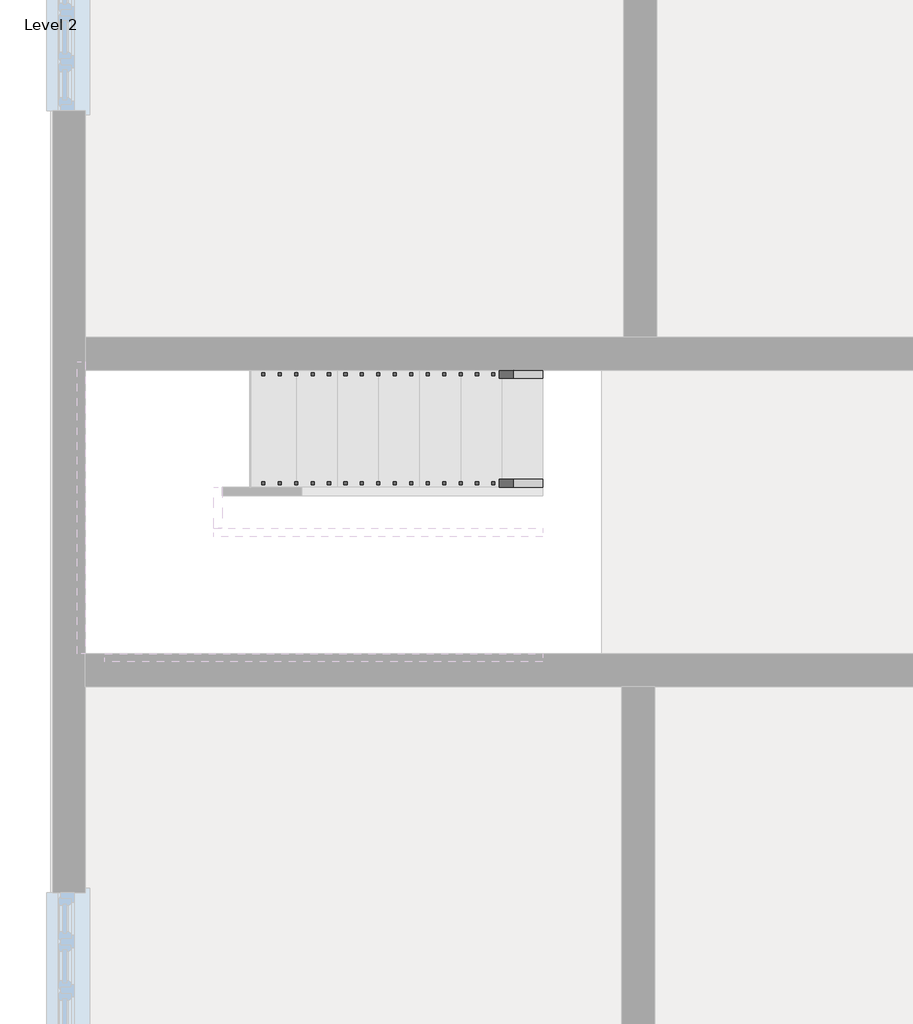
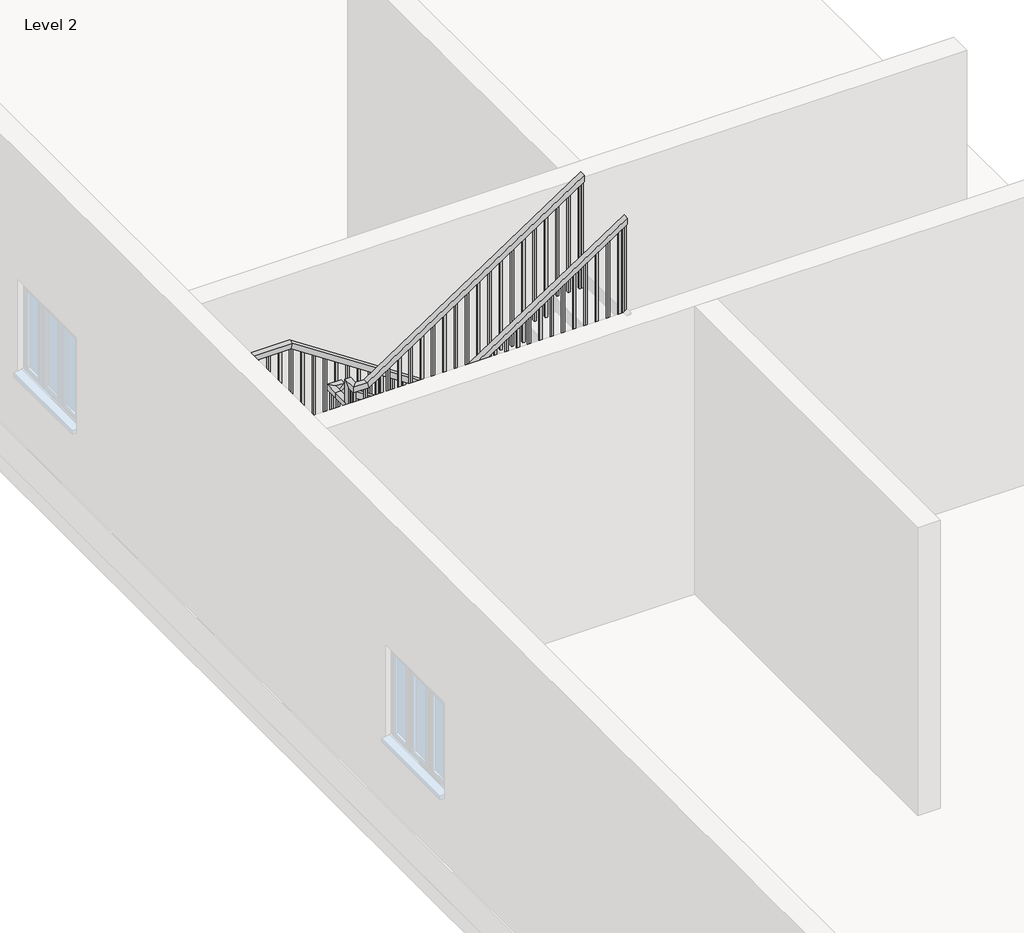
# One storey, part 2 of 3: 2 railings.
"""IFC4 building model written with IfcOpenShell, lengths in millimetres."""

from ifc_helpers import new_model, si_unit, frame, origin, place, context, project, spatial, polyline, outline, extrude, faceted_brep, element, save

model = new_model("IFC4")

# Units and contexts
model_context = context("Model", 3, world=origin())
ifc_project = project(units=[si_unit("LENGTHUNIT", "METRE", prefix="MILLI")], contexts=[model_context])

# Site, building, storey
site = spatial("IfcSite", under=ifc_project)
building = spatial("IfcBuilding", under=site)
storey = spatial("IfcBuildingStorey", under=building, Name="Level 2", Elevation=3048.0)

# Railings
placement = place(None, origin())
element("IfcRailing", 1, ObjectType="Handrail - Rectangular", at=placement, inside=storey, context=model_context, shape_type="SolidModel", body=[
    faceted_brep([(-2118.1728655, 1141.7797121, 4130.3222222), (-2118.1728655, 1141.7797121, 4069.4243166), (-2118.1728655, 1192.5797121, 4069.4243166), (-2118.1728655, 1192.5797121, 4130.3222222), (-4150.1728655, 1141.7797121, 5473.7), (-4165.4470084, 1141.7797121, 5422.9), (-4165.4470084, 1192.5797121, 5422.9), (-4150.1728655, 1192.5797121, 5473.7), (-4893.1394105, 1141.7797121, 5473.7), (-4893.1394105, 1141.7797121, 5422.9), (-4943.9394105, 1192.5797121, 5422.9), (-4943.9394105, 1192.5797121, 5473.7), (-4893.1394105, -509.2202879, 5473.7), (-4893.1394105, -509.2202879, 5422.9), (-4943.9394105, -560.0202879, 5422.9), (-4943.9394105, -560.0202879, 5473.7), (-4404.1728655, -509.2202879, 5473.7), (-4388.8987225, -509.2202879, 5422.9), (-4388.8987225, -560.0202879, 5422.9), (-4404.1728655, -560.0202879, 5473.7), (-2118.1728655, -509.2202879, 6985.0), (-2118.1728655, -560.0202879, 6985.0), (-2118.1728655, -560.0202879, 6924.1020944), (-2118.1728655, -509.2202879, 6924.1020944)], [[[0, 1, 2, 3]], [[1, 0, 4, 5]], [[2, 1, 5, 6]], [[3, 2, 6, 7]], [[0, 3, 7, 4]], [[5, 4, 8, 9]], [[6, 5, 9, 10]], [[7, 6, 10, 11]], [[4, 7, 11, 8]], [[9, 8, 12, 13]], [[10, 9, 13, 14]], [[11, 10, 14, 15]], [[8, 11, 15, 12]], [[13, 12, 16, 17]], [[14, 13, 17, 18]], [[15, 14, 18, 19]], [[12, 15, 19, 16]], [[20, 21, 22, 23]], [[17, 16, 20, 23]], [[18, 17, 23, 22]], [[19, 18, 22, 21]], [[16, 19, 21, 20]]]),
    extrude(outline(polyline([(6892.6057396, -2165.8144105), (6880.0115729, -2184.8644105), (5902.6777778, -2184.8644105), (5902.6777778, -2165.8144105), (6892.6057396, -2165.8144105)])), frame((0.0, -544.1452879, 0.0), z_axis=(0.0, 1.0, 0.0), x_axis=(0.0, 0.0, 1.0)), (0.0, 0.0, 1.0), 19.05),
    extrude(outline(polyline([(6825.4368507, -2267.4144105), (6812.842684, -2286.4644105), (5902.6777778, -2286.4644105), (5902.6777778, -2267.4144105), (6825.4368507, -2267.4144105)])), frame((0.0, -544.1452879, 0.0), z_axis=(0.0, 1.0, 0.0), x_axis=(0.0, 0.0, 1.0)), (0.0, 0.0, 1.0), 19.05),
    extrude(outline(polyline([(6758.2679618, -2369.0144105), (6745.6737951, -2388.0644105), (5734.7555556, -2388.0644105), (5734.7555556, -2369.0144105), (6758.2679618, -2369.0144105)])), frame((0.0, -544.1452879, 0.0), z_axis=(0.0, 1.0, 0.0), x_axis=(0.0, 0.0, 1.0)), (0.0, 0.0, 1.0), 19.05),
    extrude(outline(polyline([(6691.0990729, -2470.6144105), (6678.5049062, -2489.6644105), (5734.7555556, -2489.6644105), (5734.7555556, -2470.6144105), (6691.0990729, -2470.6144105)])), frame((0.0, -544.1452879, 0.0), z_axis=(0.0, 1.0, 0.0), x_axis=(0.0, 0.0, 1.0)), (0.0, 0.0, 1.0), 19.05),
    extrude(outline(polyline([(6623.930184, -2572.2144105), (6611.3360174, -2591.2644105), (5734.7555556, -2591.2644105), (5734.7555556, -2572.2144105), (6623.930184, -2572.2144105)])), frame((0.0, -544.1452879, 0.0), z_axis=(0.0, 1.0, 0.0), x_axis=(0.0, 0.0, 1.0)), (0.0, 0.0, 1.0), 19.05),
    extrude(outline(polyline([(6556.7612951, -2673.8144105), (6544.1671285, -2692.8644105), (5566.8333333, -2692.8644105), (5566.8333333, -2673.8144105), (6556.7612951, -2673.8144105)])), frame((0.0, -544.1452879, 0.0), z_axis=(0.0, 1.0, 0.0), x_axis=(0.0, 0.0, 1.0)), (0.0, 0.0, 1.0), 19.05),
    extrude(outline(polyline([(6489.5924062, -2775.4144105), (6476.9982396, -2794.4644105), (5566.8333333, -2794.4644105), (5566.8333333, -2775.4144105), (6489.5924062, -2775.4144105)])), frame((0.0, -544.1452879, 0.0), z_axis=(0.0, 1.0, 0.0), x_axis=(0.0, 0.0, 1.0)), (0.0, 0.0, 1.0), 19.05),
    extrude(outline(polyline([(6422.4235174, -2877.0144105), (6409.8293507, -2896.0644105), (5398.9111111, -2896.0644105), (5398.9111111, -2877.0144105), (6422.4235174, -2877.0144105)])), frame((0.0, -544.1452879, 0.0), z_axis=(0.0, 1.0, 0.0), x_axis=(0.0, 0.0, 1.0)), (0.0, 0.0, 1.0), 19.05),
    extrude(outline(polyline([(6355.2546285, -2978.6144105), (6342.6604618, -2997.6644105), (5398.9111111, -2997.6644105), (5398.9111111, -2978.6144105), (6355.2546285, -2978.6144105)])), frame((0.0, -544.1452879, 0.0), z_axis=(0.0, 1.0, 0.0), x_axis=(0.0, 0.0, 1.0)), (0.0, 0.0, 1.0), 19.05),
    extrude(outline(polyline([(6288.0857396, -3080.2144105), (6275.4915729, -3099.2644105), (5398.9111111, -3099.2644105), (5398.9111111, -3080.2144105), (6288.0857396, -3080.2144105)])), frame((0.0, -544.1452879, 0.0), z_axis=(0.0, 1.0, 0.0), x_axis=(0.0, 0.0, 1.0)), (0.0, 0.0, 1.0), 19.05),
    extrude(outline(polyline([(6220.9168507, -3181.8144105), (6208.322684, -3200.8644105), (5230.9888889, -3200.8644105), (5230.9888889, -3181.8144105), (6220.9168507, -3181.8144105)])), frame((0.0, -544.1452879, 0.0), z_axis=(0.0, 1.0, 0.0), x_axis=(0.0, 0.0, 1.0)), (0.0, 0.0, 1.0), 19.05),
    extrude(outline(polyline([(6153.7479618, -3283.4144105), (6141.1537951, -3302.4644105), (5230.9888889, -3302.4644105), (5230.9888889, -3283.4144105), (6153.7479618, -3283.4144105)])), frame((0.0, -544.1452879, 0.0), z_axis=(0.0, 1.0, 0.0), x_axis=(0.0, 0.0, 1.0)), (0.0, 0.0, 1.0), 19.05),
    extrude(outline(polyline([(6086.5790729, -3385.0144105), (6073.9849062, -3404.0644105), (5063.0666667, -3404.0644105), (5063.0666667, -3385.0144105), (6086.5790729, -3385.0144105)])), frame((0.0, -544.1452879, 0.0), z_axis=(0.0, 1.0, 0.0), x_axis=(0.0, 0.0, 1.0)), (0.0, 0.0, 1.0), 19.05),
    extrude(outline(polyline([(6019.410184, -3486.6144105), (6006.8160174, -3505.6644105), (5063.0666667, -3505.6644105), (5063.0666667, -3486.6144105), (6019.410184, -3486.6144105)])), frame((0.0, -544.1452879, 0.0), z_axis=(0.0, 1.0, 0.0), x_axis=(0.0, 0.0, 1.0)), (0.0, 0.0, 1.0), 19.05),
    extrude(outline(polyline([(5952.2412951, -3588.2144105), (5939.6471285, -3607.2644105), (5063.0666667, -3607.2644105), (5063.0666667, -3588.2144105), (5952.2412951, -3588.2144105)])), frame((0.0, -544.1452879, 0.0), z_axis=(0.0, 1.0, 0.0), x_axis=(0.0, 0.0, 1.0)), (0.0, 0.0, 1.0), 19.05),
    extrude(outline(polyline([(5885.0724062, -3689.8144105), (5872.4782396, -3708.8644105), (4895.1444444, -3708.8644105), (4895.1444444, -3689.8144105), (5885.0724062, -3689.8144105)])), frame((0.0, -544.1452879, 0.0), z_axis=(0.0, 1.0, 0.0), x_axis=(0.0, 0.0, 1.0)), (0.0, 0.0, 1.0), 19.05),
    extrude(outline(polyline([(5817.9035174, -3791.4144105), (5805.3093507, -3810.4644105), (4895.1444444, -3810.4644105), (4895.1444444, -3791.4144105), (5817.9035174, -3791.4144105)])), frame((0.0, -544.1452879, 0.0), z_axis=(0.0, 1.0, 0.0), x_axis=(0.0, 0.0, 1.0)), (0.0, 0.0, 1.0), 19.05),
    extrude(outline(polyline([(5750.7346285, -3893.0144105), (5738.1404618, -3912.0644105), (4727.2222222, -3912.0644105), (4727.2222222, -3893.0144105), (5750.7346285, -3893.0144105)])), frame((0.0, -544.1452879, 0.0), z_axis=(0.0, 1.0, 0.0), x_axis=(0.0, 0.0, 1.0)), (0.0, 0.0, 1.0), 19.05),
    extrude(outline(polyline([(5683.5657396, -3994.6144105), (5670.9715729, -4013.6644105), (4727.2222222, -4013.6644105), (4727.2222222, -3994.6144105), (5683.5657396, -3994.6144105)])), frame((0.0, -544.1452879, 0.0), z_axis=(0.0, 1.0, 0.0), x_axis=(0.0, 0.0, 1.0)), (0.0, 0.0, 1.0), 19.05),
    extrude(outline(polyline([(5616.3968507, -4096.2144105), (5603.802684, -4115.2644105), (4727.2222222, -4115.2644105), (4727.2222222, -4096.2144105), (5616.3968507, -4096.2144105)])), frame((0.0, -544.1452879, 0.0), z_axis=(0.0, 1.0, 0.0), x_axis=(0.0, 0.0, 1.0)), (0.0, 0.0, 1.0), 19.05),
    extrude(outline(polyline([(5549.2279618, -4197.8144105), (5536.6337951, -4216.8644105), (4559.3, -4216.8644105), (4559.3, -4197.8144105), (5549.2279618, -4197.8144105)])), frame((0.0, -544.1452879, 0.0), z_axis=(0.0, 1.0, 0.0), x_axis=(0.0, 0.0, 1.0)), (0.0, 0.0, 1.0), 19.05),
    extrude(outline(polyline([(5482.0590729, -4299.4144105), (5469.4649062, -4318.4644105), (4559.3, -4318.4644105), (4559.3, -4299.4144105), (5482.0590729, -4299.4144105)])), frame((0.0, -544.1452879, 0.0), z_axis=(0.0, 1.0, 0.0), x_axis=(0.0, 0.0, 1.0)), (0.0, 0.0, 1.0), 19.05),
    extrude(outline(polyline([(-4420.0644105, -544.1452879), (-4420.0644105, -525.0952879), (-4401.0144105, -525.0952879), (-4401.0144105, -544.1452879), (-4420.0644105, -544.1452879)])), frame((0.0, 0.0, 4559.3), z_axis=(0.0, 0.0, 1.0), x_axis=(1.0, 0.0, 0.0)), (0.0, 0.0, 1.0), 863.6),
    extrude(outline(polyline([(-4521.6644105, -544.1452879), (-4521.6644105, -525.0952879), (-4502.6144105, -525.0952879), (-4502.6144105, -544.1452879), (-4521.6644105, -544.1452879)])), frame((0.0, 0.0, 4559.3), z_axis=(0.0, 0.0, 1.0), x_axis=(1.0, 0.0, 0.0)), (0.0, 0.0, 1.0), 863.6),
    extrude(outline(polyline([(-4623.2644105, -544.1452879), (-4623.2644105, -525.0952879), (-4604.2144105, -525.0952879), (-4604.2144105, -544.1452879), (-4623.2644105, -544.1452879)])), frame((0.0, 0.0, 4559.3), z_axis=(0.0, 0.0, 1.0), x_axis=(1.0, 0.0, 0.0)), (0.0, 0.0, 1.0), 863.6),
    extrude(outline(polyline([(-4724.8644105, -544.1452879), (-4724.8644105, -525.0952879), (-4705.8144105, -525.0952879), (-4705.8144105, -544.1452879), (-4724.8644105, -544.1452879)])), frame((0.0, 0.0, 4559.3), z_axis=(0.0, 0.0, 1.0), x_axis=(1.0, 0.0, 0.0)), (0.0, 0.0, 1.0), 863.6),
    extrude(outline(polyline([(-4826.4644105, -544.1452879), (-4826.4644105, -525.0952879), (-4807.4144105, -525.0952879), (-4807.4144105, -544.1452879), (-4826.4644105, -544.1452879)])), frame((0.0, 0.0, 4559.3), z_axis=(0.0, 0.0, 1.0), x_axis=(1.0, 0.0, 0.0)), (0.0, 0.0, 1.0), 863.6),
    extrude(outline(polyline([(-4928.0644105, -448.8952879), (-4909.0144105, -448.8952879), (-4909.0144105, -467.9452879), (-4928.0644105, -467.9452879), (-4928.0644105, -448.8952879)])), frame((0.0, 0.0, 4559.3), z_axis=(0.0, 0.0, 1.0), x_axis=(1.0, 0.0, 0.0)), (0.0, 0.0, 1.0), 863.6),
    extrude(outline(polyline([(-4928.0644105, -347.2952879), (-4909.0144105, -347.2952879), (-4909.0144105, -366.3452879), (-4928.0644105, -366.3452879), (-4928.0644105, -347.2952879)])), frame((0.0, 0.0, 4559.3), z_axis=(0.0, 0.0, 1.0), x_axis=(1.0, 0.0, 0.0)), (0.0, 0.0, 1.0), 863.6),
    extrude(outline(polyline([(-4928.0644105, -245.6952879), (-4909.0144105, -245.6952879), (-4909.0144105, -264.7452879), (-4928.0644105, -264.7452879), (-4928.0644105, -245.6952879)])), frame((0.0, 0.0, 4559.3), z_axis=(0.0, 0.0, 1.0), x_axis=(1.0, 0.0, 0.0)), (0.0, 0.0, 1.0), 863.6),
    extrude(outline(polyline([(-4928.0644105, -144.0952879), (-4909.0144105, -144.0952879), (-4909.0144105, -163.1452879), (-4928.0644105, -163.1452879), (-4928.0644105, -144.0952879)])), frame((0.0, 0.0, 4559.3), z_axis=(0.0, 0.0, 1.0), x_axis=(1.0, 0.0, 0.0)), (0.0, 0.0, 1.0), 863.6),
    extrude(outline(polyline([(-4928.0644105, -42.4952879), (-4909.0144105, -42.4952879), (-4909.0144105, -61.5452879), (-4928.0644105, -61.5452879), (-4928.0644105, -42.4952879)])), frame((0.0, 0.0, 4559.3), z_axis=(0.0, 0.0, 1.0), x_axis=(1.0, 0.0, 0.0)), (0.0, 0.0, 1.0), 863.6),
    extrude(outline(polyline([(-4928.0644105, 59.1047121), (-4909.0144105, 59.1047121), (-4909.0144105, 40.0547121), (-4928.0644105, 40.0547121), (-4928.0644105, 59.1047121)])), frame((0.0, 0.0, 4559.3), z_axis=(0.0, 0.0, 1.0), x_axis=(1.0, 0.0, 0.0)), (0.0, 0.0, 1.0), 863.6),
    extrude(outline(polyline([(-4928.0644105, 160.7047121), (-4909.0144105, 160.7047121), (-4909.0144105, 141.6547121), (-4928.0644105, 141.6547121), (-4928.0644105, 160.7047121)])), frame((0.0, 0.0, 4559.3), z_axis=(0.0, 0.0, 1.0), x_axis=(1.0, 0.0, 0.0)), (0.0, 0.0, 1.0), 863.6),
    extrude(outline(polyline([(-4928.0644105, 262.3047121), (-4909.0144105, 262.3047121), (-4909.0144105, 243.2547121), (-4928.0644105, 243.2547121), (-4928.0644105, 262.3047121)])), frame((0.0, 0.0, 4559.3), z_axis=(0.0, 0.0, 1.0), x_axis=(1.0, 0.0, 0.0)), (0.0, 0.0, 1.0), 863.6),
    extrude(outline(polyline([(-4928.0644105, 363.9047121), (-4909.0144105, 363.9047121), (-4909.0144105, 344.8547121), (-4928.0644105, 344.8547121), (-4928.0644105, 363.9047121)])), frame((0.0, 0.0, 4559.3), z_axis=(0.0, 0.0, 1.0), x_axis=(1.0, 0.0, 0.0)), (0.0, 0.0, 1.0), 863.6),
    extrude(outline(polyline([(-4928.0644105, 465.5047121), (-4909.0144105, 465.5047121), (-4909.0144105, 446.4547121), (-4928.0644105, 446.4547121), (-4928.0644105, 465.5047121)])), frame((0.0, 0.0, 4559.3), z_axis=(0.0, 0.0, 1.0), x_axis=(1.0, 0.0, 0.0)), (0.0, 0.0, 1.0), 863.6),
    extrude(outline(polyline([(-4928.0644105, 567.1047121), (-4909.0144105, 567.1047121), (-4909.0144105, 548.0547121), (-4928.0644105, 548.0547121), (-4928.0644105, 567.1047121)])), frame((0.0, 0.0, 4559.3), z_axis=(0.0, 0.0, 1.0), x_axis=(1.0, 0.0, 0.0)), (0.0, 0.0, 1.0), 863.6),
    extrude(outline(polyline([(-4928.0644105, 668.7047121), (-4909.0144105, 668.7047121), (-4909.0144105, 649.6547121), (-4928.0644105, 649.6547121), (-4928.0644105, 668.7047121)])), frame((0.0, 0.0, 4559.3), z_axis=(0.0, 0.0, 1.0), x_axis=(1.0, 0.0, 0.0)), (0.0, 0.0, 1.0), 863.6),
    extrude(outline(polyline([(-4928.0644105, 770.3047121), (-4909.0144105, 770.3047121), (-4909.0144105, 751.2547121), (-4928.0644105, 751.2547121), (-4928.0644105, 770.3047121)])), frame((0.0, 0.0, 4559.3), z_axis=(0.0, 0.0, 1.0), x_axis=(1.0, 0.0, 0.0)), (0.0, 0.0, 1.0), 863.6),
    extrude(outline(polyline([(-4928.0644105, 871.9047121), (-4909.0144105, 871.9047121), (-4909.0144105, 852.8547121), (-4928.0644105, 852.8547121), (-4928.0644105, 871.9047121)])), frame((0.0, 0.0, 4559.3), z_axis=(0.0, 0.0, 1.0), x_axis=(1.0, 0.0, 0.0)), (0.0, 0.0, 1.0), 863.6),
    extrude(outline(polyline([(-4928.0644105, 973.5047121), (-4909.0144105, 973.5047121), (-4909.0144105, 954.4547121), (-4928.0644105, 954.4547121), (-4928.0644105, 973.5047121)])), frame((0.0, 0.0, 4559.3), z_axis=(0.0, 0.0, 1.0), x_axis=(1.0, 0.0, 0.0)), (0.0, 0.0, 1.0), 863.6),
    extrude(outline(polyline([(-4928.0644105, 1075.1047121), (-4909.0144105, 1075.1047121), (-4909.0144105, 1056.0547121), (-4928.0644105, 1056.0547121), (-4928.0644105, 1075.1047121)])), frame((0.0, 0.0, 4559.3), z_axis=(0.0, 0.0, 1.0), x_axis=(1.0, 0.0, 0.0)), (0.0, 0.0, 1.0), 863.6),
    extrude(outline(polyline([(-4851.8478655, 1176.7047121), (-4851.8478655, 1157.6547121), (-4870.8978655, 1157.6547121), (-4870.8978655, 1176.7047121), (-4851.8478655, 1176.7047121)])), frame((0.0, 0.0, 4559.3), z_axis=(0.0, 0.0, 1.0), x_axis=(1.0, 0.0, 0.0)), (0.0, 0.0, 1.0), 863.6),
    extrude(outline(polyline([(-4750.2478655, 1176.7047121), (-4750.2478655, 1157.6547121), (-4769.2978655, 1157.6547121), (-4769.2978655, 1176.7047121), (-4750.2478655, 1176.7047121)])), frame((0.0, 0.0, 4559.3), z_axis=(0.0, 0.0, 1.0), x_axis=(1.0, 0.0, 0.0)), (0.0, 0.0, 1.0), 863.6),
    extrude(outline(polyline([(-4648.6478655, 1176.7047121), (-4648.6478655, 1157.6547121), (-4667.6978655, 1157.6547121), (-4667.6978655, 1176.7047121), (-4648.6478655, 1176.7047121)])), frame((0.0, 0.0, 4559.3), z_axis=(0.0, 0.0, 1.0), x_axis=(1.0, 0.0, 0.0)), (0.0, 0.0, 1.0), 863.6),
    extrude(outline(polyline([(-4547.0478655, 1176.7047121), (-4547.0478655, 1157.6547121), (-4566.0978655, 1157.6547121), (-4566.0978655, 1176.7047121), (-4547.0478655, 1176.7047121)])), frame((0.0, 0.0, 4559.3), z_axis=(0.0, 0.0, 1.0), x_axis=(1.0, 0.0, 0.0)), (0.0, 0.0, 1.0), 863.6),
    extrude(outline(polyline([(-4445.4478655, 1176.7047121), (-4445.4478655, 1157.6547121), (-4464.4978655, 1157.6547121), (-4464.4978655, 1176.7047121), (-4445.4478655, 1176.7047121)])), frame((0.0, 0.0, 4559.3), z_axis=(0.0, 0.0, 1.0), x_axis=(1.0, 0.0, 0.0)), (0.0, 0.0, 1.0), 863.6),
    extrude(outline(polyline([(-4343.8478655, 1176.7047121), (-4343.8478655, 1157.6547121), (-4362.8978655, 1157.6547121), (-4362.8978655, 1176.7047121), (-4343.8478655, 1176.7047121)])), frame((0.0, 0.0, 4559.3), z_axis=(0.0, 0.0, 1.0), x_axis=(1.0, 0.0, 0.0)), (0.0, 0.0, 1.0), 863.6),
    extrude(outline(polyline([(-4242.2478655, 1176.7047121), (-4242.2478655, 1157.6547121), (-4261.2978655, 1157.6547121), (-4261.2978655, 1176.7047121), (-4242.2478655, 1176.7047121)])), frame((0.0, 0.0, 4559.3), z_axis=(0.0, 0.0, 1.0), x_axis=(1.0, 0.0, 0.0)), (0.0, 0.0, 1.0), 863.6),
    extrude(outline(polyline([(5406.505011, -4140.6478655), (5419.0991777, -4159.6978655), (4559.3, -4159.6978655), (4559.3, -4140.6478655), (5406.505011, -4140.6478655)])), frame((0.0, 1157.6547121, 0.0), z_axis=(0.0, 1.0, 0.0), x_axis=(0.0, 0.0, 1.0)), (0.0, 0.0, 1.0), 19.05),
    extrude(outline(polyline([(5339.3361222, -4039.0478655), (5351.9302888, -4058.0978655), (4391.3777778, -4058.0978655), (4391.3777778, -4039.0478655), (5339.3361222, -4039.0478655)])), frame((0.0, 1157.6547121, 0.0), z_axis=(0.0, 1.0, 0.0), x_axis=(0.0, 0.0, 1.0)), (0.0, 0.0, 1.0), 19.05),
    extrude(outline(polyline([(5272.1672333, -3937.4478655), (5284.7613999, -3956.4978655), (4391.3777778, -3956.4978655), (4391.3777778, -3937.4478655), (5272.1672333, -3937.4478655)])), frame((0.0, 1157.6547121, 0.0), z_axis=(0.0, 1.0, 0.0), x_axis=(0.0, 0.0, 1.0)), (0.0, 0.0, 1.0), 19.05),
    extrude(outline(polyline([(5204.9983444, -3835.8478655), (5217.592511, -3854.8978655), (4223.4555556, -3854.8978655), (4223.4555556, -3835.8478655), (5204.9983444, -3835.8478655)])), frame((0.0, 1157.6547121, 0.0), z_axis=(0.0, 1.0, 0.0), x_axis=(0.0, 0.0, 1.0)), (0.0, 0.0, 1.0), 19.05),
    extrude(outline(polyline([(5137.8294555, -3734.2478655), (5150.4236222, -3753.2978655), (4223.4555556, -3753.2978655), (4223.4555556, -3734.2478655), (5137.8294555, -3734.2478655)])), frame((0.0, 1157.6547121, 0.0), z_axis=(0.0, 1.0, 0.0), x_axis=(0.0, 0.0, 1.0)), (0.0, 0.0, 1.0), 19.05),
    extrude(outline(polyline([(5070.6605666, -3632.6478655), (5083.2547333, -3651.6978655), (4223.4555556, -3651.6978655), (4223.4555556, -3632.6478655), (5070.6605666, -3632.6478655)])), frame((0.0, 1157.6547121, 0.0), z_axis=(0.0, 1.0, 0.0), x_axis=(0.0, 0.0, 1.0)), (0.0, 0.0, 1.0), 19.05),
    extrude(outline(polyline([(5003.4916777, -3531.0478655), (5016.0858444, -3550.0978655), (4055.5333333, -3550.0978655), (4055.5333333, -3531.0478655), (5003.4916777, -3531.0478655)])), frame((0.0, 1157.6547121, 0.0), z_axis=(0.0, 1.0, 0.0), x_axis=(0.0, 0.0, 1.0)), (0.0, 0.0, 1.0), 19.05),
    extrude(outline(polyline([(4936.3227888, -3429.4478655), (4948.9169555, -3448.4978655), (4055.5333333, -3448.4978655), (4055.5333333, -3429.4478655), (4936.3227888, -3429.4478655)])), frame((0.0, 1157.6547121, 0.0), z_axis=(0.0, 1.0, 0.0), x_axis=(0.0, 0.0, 1.0)), (0.0, 0.0, 1.0), 19.05),
    extrude(outline(polyline([(4869.1538999, -3327.8478655), (4881.7480666, -3346.8978655), (3887.6111111, -3346.8978655), (3887.6111111, -3327.8478655), (4869.1538999, -3327.8478655)])), frame((0.0, 1157.6547121, 0.0), z_axis=(0.0, 1.0, 0.0), x_axis=(0.0, 0.0, 1.0)), (0.0, 0.0, 1.0), 19.05),
    extrude(outline(polyline([(4801.985011, -3226.2478655), (4814.5791777, -3245.2978655), (3887.6111111, -3245.2978655), (3887.6111111, -3226.2478655), (4801.985011, -3226.2478655)])), frame((0.0, 1157.6547121, 0.0), z_axis=(0.0, 1.0, 0.0), x_axis=(0.0, 0.0, 1.0)), (0.0, 0.0, 1.0), 19.05),
    extrude(outline(polyline([(4734.8161222, -3124.6478655), (4747.4102888, -3143.6978655), (3887.6111111, -3143.6978655), (3887.6111111, -3124.6478655), (4734.8161222, -3124.6478655)])), frame((0.0, 1157.6547121, 0.0), z_axis=(0.0, 1.0, 0.0), x_axis=(0.0, 0.0, 1.0)), (0.0, 0.0, 1.0), 19.05),
    extrude(outline(polyline([(4667.6472333, -3023.0478655), (4680.2413999, -3042.0978655), (3719.6888889, -3042.0978655), (3719.6888889, -3023.0478655), (4667.6472333, -3023.0478655)])), frame((0.0, 1157.6547121, 0.0), z_axis=(0.0, 1.0, 0.0), x_axis=(0.0, 0.0, 1.0)), (0.0, 0.0, 1.0), 19.05),
    extrude(outline(polyline([(4600.4783444, -2921.4478655), (4613.072511, -2940.4978655), (3719.6888889, -2940.4978655), (3719.6888889, -2921.4478655), (4600.4783444, -2921.4478655)])), frame((0.0, 1157.6547121, 0.0), z_axis=(0.0, 1.0, 0.0), x_axis=(0.0, 0.0, 1.0)), (0.0, 0.0, 1.0), 19.05),
    extrude(outline(polyline([(4533.3094555, -2819.8478655), (4545.9036222, -2838.8978655), (3551.7666667, -2838.8978655), (3551.7666667, -2819.8478655), (4533.3094555, -2819.8478655)])), frame((0.0, 1157.6547121, 0.0), z_axis=(0.0, 1.0, 0.0), x_axis=(0.0, 0.0, 1.0)), (0.0, 0.0, 1.0), 19.05),
    extrude(outline(polyline([(4466.1405666, -2718.2478655), (4478.7347333, -2737.2978655), (3551.7666667, -2737.2978655), (3551.7666667, -2718.2478655), (4466.1405666, -2718.2478655)])), frame((0.0, 1157.6547121, 0.0), z_axis=(0.0, 1.0, 0.0), x_axis=(0.0, 0.0, 1.0)), (0.0, 0.0, 1.0), 19.05),
    extrude(outline(polyline([(4398.9716777, -2616.6478655), (4411.5658444, -2635.6978655), (3551.7666667, -2635.6978655), (3551.7666667, -2616.6478655), (4398.9716777, -2616.6478655)])), frame((0.0, 1157.6547121, 0.0), z_axis=(0.0, 1.0, 0.0), x_axis=(0.0, 0.0, 1.0)), (0.0, 0.0, 1.0), 19.05),
    extrude(outline(polyline([(4331.8027888, -2515.0478655), (4344.3969555, -2534.0978655), (3383.8444444, -2534.0978655), (3383.8444444, -2515.0478655), (4331.8027888, -2515.0478655)])), frame((0.0, 1157.6547121, 0.0), z_axis=(0.0, 1.0, 0.0), x_axis=(0.0, 0.0, 1.0)), (0.0, 0.0, 1.0), 19.05),
    extrude(outline(polyline([(4264.6338999, -2413.4478655), (4277.2280666, -2432.4978655), (3383.8444444, -2432.4978655), (3383.8444444, -2413.4478655), (4264.6338999, -2413.4478655)])), frame((0.0, 1157.6547121, 0.0), z_axis=(0.0, 1.0, 0.0), x_axis=(0.0, 0.0, 1.0)), (0.0, 0.0, 1.0), 19.05),
    extrude(outline(polyline([(4197.465011, -2311.8478655), (4210.0591777, -2330.8978655), (3215.9222222, -2330.8978655), (3215.9222222, -2311.8478655), (4197.465011, -2311.8478655)])), frame((0.0, 1157.6547121, 0.0), z_axis=(0.0, 1.0, 0.0), x_axis=(0.0, 0.0, 1.0)), (0.0, 0.0, 1.0), 19.05),
    extrude(outline(polyline([(4130.2961222, -2210.2478655), (4142.8902888, -2229.2978655), (3215.9222222, -2229.2978655), (3215.9222222, -2210.2478655), (4130.2961222, -2210.2478655)])), frame((0.0, 1157.6547121, 0.0), z_axis=(0.0, 1.0, 0.0), x_axis=(0.0, 0.0, 1.0)), (0.0, 0.0, 1.0), 19.05),
    extrude(outline(polyline([(-4928.0644105, -525.0952879), (-4909.0144105, -525.0952879), (-4909.0144105, -544.1452879), (-4928.0644105, -544.1452879), (-4928.0644105, -525.0952879)])), frame((0.0, 0.0, 4559.3), z_axis=(0.0, 0.0, 1.0), x_axis=(1.0, 0.0, 0.0)), (0.0, 0.0, 1.0), 863.6),
    extrude(outline(polyline([(-4909.0144105, 1176.7047121), (-4909.0144105, 1157.6547121), (-4928.0644105, 1157.6547121), (-4928.0644105, 1176.7047121), (-4909.0144105, 1176.7047121)])), frame((0.0, 0.0, 4559.3), z_axis=(0.0, 0.0, 1.0), x_axis=(1.0, 0.0, 0.0)), (0.0, 0.0, 1.0), 863.6),
    extrude(outline(polyline([(6924.1020944, -2118.1728655), (6911.5079277, -2137.2228655), (5902.6777778, -2137.2228655), (5902.6777778, -2118.1728655), (6924.1020944, -2118.1728655)])), frame((0.0, -544.1452879, 0.0), z_axis=(0.0, 1.0, 0.0), x_axis=(0.0, 0.0, 1.0)), (0.0, 0.0, 1.0), 19.05),
    extrude(outline(polyline([(4069.4243166, -2118.1728655), (4082.0184833, -2137.2228655), (3215.9222222, -2137.2228655), (3215.9222222, -2118.1728655), (4069.4243166, -2118.1728655)])), frame((0.0, 1157.6547121, 0.0), z_axis=(0.0, 1.0, 0.0), x_axis=(0.0, 0.0, 1.0)), (0.0, 0.0, 1.0), 19.05),
])
element("IfcRailing", 2, ObjectType="Handrail - Rectangular", at=placement, inside=storey, context=model_context, shape_type="SolidModel", body=[
    faceted_brep([(-2118.1728655, 468.6797121, 4130.3222222), (-2118.1728655, 468.6797121, 4069.4243166), (-2118.1728655, 519.4797121, 4069.4243166), (-2118.1728655, 519.4797121, 4130.3222222), (-4073.9728655, 468.6797121, 5423.3233333), (-4124.7728655, 468.6797121, 5396.0098722), (-4124.7728655, 519.4797121, 5396.0098722), (-4073.9728655, 519.4797121, 5423.3233333), (-4073.9728655, 468.6797121, 5473.7), (-4124.7728655, 468.6797121, 5422.9), (-4124.7728655, 519.4797121, 5422.9), (-4073.9728655, 519.4797121, 5473.7), (-4150.1728655, 468.6797121, 5473.7), (-4150.1728655, 468.6797121, 5422.9), (-4200.9728655, 519.4797121, 5422.9), (-4200.9728655, 519.4797121, 5473.7), (-4150.1728655, 392.4797121, 5473.7), (-4150.1728655, 392.4797121, 5422.9), (-4200.9728655, 392.4797121, 5422.9), (-4200.9728655, 392.4797121, 5473.7), (-4150.1728655, 240.0797121, 5473.7), (-4150.1728655, 189.2797121, 5422.9), (-4200.9728655, 189.2797121, 5422.9), (-4200.9728655, 240.0797121, 5473.7), (-4150.1728655, 240.0797121, 5691.9988889), (-4150.1728655, 189.2797121, 5641.1988889), (-4200.9728655, 189.2797121, 5641.1988889), (-4200.9728655, 240.0797121, 5691.9988889), (-4150.1728655, 163.8797121, 5691.9988889), (-4150.1728655, 163.8797121, 5641.1988889), (-4200.9728655, 113.0797121, 5641.1988889), (-4200.9728655, 113.0797121, 5691.9988889), (-4073.9728655, 163.8797121, 5691.9988889), (-4058.6987225, 163.8797121, 5641.1988889), (-4058.6987225, 113.0797121, 5641.1988889), (-4073.9728655, 113.0797121, 5691.9988889), (-2118.1728655, 163.8797121, 6985.0), (-2118.1728655, 113.0797121, 6985.0), (-2118.1728655, 113.0797121, 6924.1020944), (-2118.1728655, 163.8797121, 6924.1020944)], [[[0, 1, 2, 3]], [[1, 0, 4, 5]], [[2, 1, 5, 6]], [[3, 2, 6, 7]], [[0, 3, 7, 4]], [[5, 4, 8, 9]], [[6, 5, 9, 10]], [[7, 6, 10, 11]], [[4, 7, 11, 8]], [[9, 8, 12, 13]], [[10, 9, 13, 14]], [[11, 10, 14, 15]], [[8, 11, 15, 12]], [[13, 12, 16, 17]], [[14, 13, 17, 18]], [[15, 14, 18, 19]], [[12, 15, 19, 16]], [[17, 16, 20, 21]], [[18, 17, 21, 22]], [[19, 18, 22, 23]], [[16, 19, 23, 20]], [[21, 20, 24, 25]], [[22, 21, 25, 26]], [[23, 22, 26, 27]], [[20, 23, 27, 24]], [[25, 24, 28, 29]], [[26, 25, 29, 30]], [[27, 26, 30, 31]], [[24, 27, 31, 28]], [[29, 28, 32, 33]], [[30, 29, 33, 34]], [[31, 30, 34, 35]], [[28, 31, 35, 32]], [[36, 37, 38, 39]], [[33, 32, 36, 39]], [[34, 33, 39, 38]], [[35, 34, 38, 37]], [[32, 35, 37, 36]]]),
    extrude(outline(polyline([(6901.0127888, -2153.0978655), (5902.6777778, -2153.0978655), (5902.6777778, -2134.0478655), (6913.6069555, -2134.0478655), (6901.0127888, -2153.0978655)])), frame((0.0, 128.9547121, 0.0), z_axis=(0.0, 1.0, 0.0), x_axis=(0.0, 0.0, 1.0)), (0.0, 0.0, 1.0), 19.05),
    extrude(outline(polyline([(6833.8438999, -2254.6978655), (5902.6777778, -2254.6978655), (5902.6777778, -2235.6478655), (6846.4380666, -2235.6478655), (6833.8438999, -2254.6978655)])), frame((0.0, 128.9547121, 0.0), z_axis=(0.0, 1.0, 0.0), x_axis=(0.0, 0.0, 1.0)), (0.0, 0.0, 1.0), 19.05),
    extrude(outline(polyline([(6766.675011, -2356.2978655), (5902.6777778, -2356.2978655), (5902.6777778, -2337.2478655), (6779.2691777, -2337.2478655), (6766.675011, -2356.2978655)])), frame((0.0, 128.9547121, 0.0), z_axis=(0.0, 1.0, 0.0), x_axis=(0.0, 0.0, 1.0)), (0.0, 0.0, 1.0), 19.05),
    extrude(outline(polyline([(6699.5061222, -2457.8978655), (5734.7555556, -2457.8978655), (5734.7555556, -2438.8478655), (6712.1002888, -2438.8478655), (6699.5061222, -2457.8978655)])), frame((0.0, 128.9547121, 0.0), z_axis=(0.0, 1.0, 0.0), x_axis=(0.0, 0.0, 1.0)), (0.0, 0.0, 1.0), 19.05),
    extrude(outline(polyline([(6632.3372333, -2559.4978655), (5734.7555556, -2559.4978655), (5734.7555556, -2540.4478655), (6644.9313999, -2540.4478655), (6632.3372333, -2559.4978655)])), frame((0.0, 128.9547121, 0.0), z_axis=(0.0, 1.0, 0.0), x_axis=(0.0, 0.0, 1.0)), (0.0, 0.0, 1.0), 19.05),
    extrude(outline(polyline([(6565.1683444, -2661.0978655), (5566.8333333, -2661.0978655), (5566.8333333, -2642.0478655), (6577.762511, -2642.0478655), (6565.1683444, -2661.0978655)])), frame((0.0, 128.9547121, 0.0), z_axis=(0.0, 1.0, 0.0), x_axis=(0.0, 0.0, 1.0)), (0.0, 0.0, 1.0), 19.05),
    extrude(outline(polyline([(6497.9994555, -2762.6978655), (5566.8333333, -2762.6978655), (5566.8333333, -2743.6478655), (6510.5936222, -2743.6478655), (6497.9994555, -2762.6978655)])), frame((0.0, 128.9547121, 0.0), z_axis=(0.0, 1.0, 0.0), x_axis=(0.0, 0.0, 1.0)), (0.0, 0.0, 1.0), 19.05),
    extrude(outline(polyline([(6430.8305666, -2864.2978655), (5566.8333333, -2864.2978655), (5566.8333333, -2845.2478655), (6443.4247333, -2845.2478655), (6430.8305666, -2864.2978655)])), frame((0.0, 128.9547121, 0.0), z_axis=(0.0, 1.0, 0.0), x_axis=(0.0, 0.0, 1.0)), (0.0, 0.0, 1.0), 19.05),
    extrude(outline(polyline([(6363.6616777, -2965.8978655), (5398.9111111, -2965.8978655), (5398.9111111, -2946.8478655), (6376.2558444, -2946.8478655), (6363.6616777, -2965.8978655)])), frame((0.0, 128.9547121, 0.0), z_axis=(0.0, 1.0, 0.0), x_axis=(0.0, 0.0, 1.0)), (0.0, 0.0, 1.0), 19.05),
    extrude(outline(polyline([(6296.4927888, -3067.4978655), (5398.9111111, -3067.4978655), (5398.9111111, -3048.4478655), (6309.0869555, -3048.4478655), (6296.4927888, -3067.4978655)])), frame((0.0, 128.9547121, 0.0), z_axis=(0.0, 1.0, 0.0), x_axis=(0.0, 0.0, 1.0)), (0.0, 0.0, 1.0), 19.05),
    extrude(outline(polyline([(6229.3238999, -3169.0978655), (5230.9888889, -3169.0978655), (5230.9888889, -3150.0478655), (6241.9180666, -3150.0478655), (6229.3238999, -3169.0978655)])), frame((0.0, 128.9547121, 0.0), z_axis=(0.0, 1.0, 0.0), x_axis=(0.0, 0.0, 1.0)), (0.0, 0.0, 1.0), 19.05),
    extrude(outline(polyline([(6162.155011, -3270.6978655), (5230.9888889, -3270.6978655), (5230.9888889, -3251.6478655), (6174.7491777, -3251.6478655), (6162.155011, -3270.6978655)])), frame((0.0, 128.9547121, 0.0), z_axis=(0.0, 1.0, 0.0), x_axis=(0.0, 0.0, 1.0)), (0.0, 0.0, 1.0), 19.05),
    extrude(outline(polyline([(6094.9861222, -3372.2978655), (5230.9888889, -3372.2978655), (5230.9888889, -3353.2478655), (6107.5802888, -3353.2478655), (6094.9861222, -3372.2978655)])), frame((0.0, 128.9547121, 0.0), z_axis=(0.0, 1.0, 0.0), x_axis=(0.0, 0.0, 1.0)), (0.0, 0.0, 1.0), 19.05),
    extrude(outline(polyline([(6027.8172333, -3473.8978655), (5063.0666667, -3473.8978655), (5063.0666667, -3454.8478655), (6040.4113999, -3454.8478655), (6027.8172333, -3473.8978655)])), frame((0.0, 128.9547121, 0.0), z_axis=(0.0, 1.0, 0.0), x_axis=(0.0, 0.0, 1.0)), (0.0, 0.0, 1.0), 19.05),
    extrude(outline(polyline([(5960.6483444, -3575.4978655), (5063.0666667, -3575.4978655), (5063.0666667, -3556.4478655), (5973.242511, -3556.4478655), (5960.6483444, -3575.4978655)])), frame((0.0, 128.9547121, 0.0), z_axis=(0.0, 1.0, 0.0), x_axis=(0.0, 0.0, 1.0)), (0.0, 0.0, 1.0), 19.05),
    extrude(outline(polyline([(5893.4794555, -3677.0978655), (4895.1444444, -3677.0978655), (4895.1444444, -3658.0478655), (5906.0736222, -3658.0478655), (5893.4794555, -3677.0978655)])), frame((0.0, 128.9547121, 0.0), z_axis=(0.0, 1.0, 0.0), x_axis=(0.0, 0.0, 1.0)), (0.0, 0.0, 1.0), 19.05),
    extrude(outline(polyline([(5826.3105666, -3778.6978655), (4895.1444444, -3778.6978655), (4895.1444444, -3759.6478655), (5838.9047333, -3759.6478655), (5826.3105666, -3778.6978655)])), frame((0.0, 128.9547121, 0.0), z_axis=(0.0, 1.0, 0.0), x_axis=(0.0, 0.0, 1.0)), (0.0, 0.0, 1.0), 19.05),
    extrude(outline(polyline([(5759.1416777, -3880.2978655), (4895.1444444, -3880.2978655), (4895.1444444, -3861.2478655), (5771.7358444, -3861.2478655), (5759.1416777, -3880.2978655)])), frame((0.0, 128.9547121, 0.0), z_axis=(0.0, 1.0, 0.0), x_axis=(0.0, 0.0, 1.0)), (0.0, 0.0, 1.0), 19.05),
    extrude(outline(polyline([(5691.9727888, -3981.8978655), (4727.2222222, -3981.8978655), (4727.2222222, -3962.8478655), (5704.5669555, -3962.8478655), (5691.9727888, -3981.8978655)])), frame((0.0, 128.9547121, 0.0), z_axis=(0.0, 1.0, 0.0), x_axis=(0.0, 0.0, 1.0)), (0.0, 0.0, 1.0), 19.05),
    extrude(outline(polyline([(5624.8038999, -4083.4978655), (4727.2222222, -4083.4978655), (4727.2222222, -4064.4478655), (5637.3980666, -4064.4478655), (5624.8038999, -4083.4978655)])), frame((0.0, 128.9547121, 0.0), z_axis=(0.0, 1.0, 0.0), x_axis=(0.0, 0.0, 1.0)), (0.0, 0.0, 1.0), 19.05),
    extrude(outline(polyline([(-4166.0478655, 198.8047121), (-4166.0478655, 179.7547121), (-4185.0978655, 179.7547121), (-4185.0978655, 198.8047121), (-4166.0478655, 198.8047121)])), frame((0.0, 0.0, 4559.3), z_axis=(0.0, 0.0, 1.0), x_axis=(1.0, 0.0, 0.0)), (0.0, 0.0, 1.0), 1081.8988889),
    extrude(outline(polyline([(-4166.0478655, 300.4047121), (-4166.0478655, 281.3547121), (-4185.0978655, 281.3547121), (-4185.0978655, 300.4047121), (-4166.0478655, 300.4047121)])), frame((0.0, 0.0, 4559.3), z_axis=(0.0, 0.0, 1.0), x_axis=(1.0, 0.0, 0.0)), (0.0, 0.0, 1.0), 863.6),
    extrude(outline(polyline([(-4166.0478655, 402.0047121), (-4166.0478655, 382.9547121), (-4185.0978655, 382.9547121), (-4185.0978655, 402.0047121), (-4166.0478655, 402.0047121)])), frame((0.0, 0.0, 4559.3), z_axis=(0.0, 0.0, 1.0), x_axis=(1.0, 0.0, 0.0)), (0.0, 0.0, 1.0), 863.6),
    extrude(outline(polyline([(-4140.6478655, 484.5547121), (-4159.6978655, 484.5547121), (-4159.6978655, 503.6047121), (-4140.6478655, 503.6047121), (-4140.6478655, 484.5547121)])), frame((0.0, 0.0, 4559.3), z_axis=(0.0, 0.0, 1.0), x_axis=(1.0, 0.0, 0.0)), (0.0, 0.0, 1.0), 863.6),
    extrude(outline(polyline([(5351.9302888, -4058.0978655), (4391.3777778, -4058.0978655), (4391.3777778, -4039.0478655), (5339.3361222, -4039.0478655), (5351.9302888, -4058.0978655)])), frame((0.0, 484.5547121, 0.0), z_axis=(0.0, 1.0, 0.0), x_axis=(0.0, 0.0, 1.0)), (0.0, 0.0, 1.0), 19.05),
    extrude(outline(polyline([(5284.7613999, -3956.4978655), (4391.3777778, -3956.4978655), (4391.3777778, -3937.4478655), (5272.1672333, -3937.4478655), (5284.7613999, -3956.4978655)])), frame((0.0, 484.5547121, 0.0), z_axis=(0.0, 1.0, 0.0), x_axis=(0.0, 0.0, 1.0)), (0.0, 0.0, 1.0), 19.05),
    extrude(outline(polyline([(5217.592511, -3854.8978655), (4223.4555556, -3854.8978655), (4223.4555556, -3835.8478655), (5204.9983444, -3835.8478655), (5217.592511, -3854.8978655)])), frame((0.0, 484.5547121, 0.0), z_axis=(0.0, 1.0, 0.0), x_axis=(0.0, 0.0, 1.0)), (0.0, 0.0, 1.0), 19.05),
    extrude(outline(polyline([(5150.4236222, -3753.2978655), (4223.4555556, -3753.2978655), (4223.4555556, -3734.2478655), (5137.8294555, -3734.2478655), (5150.4236222, -3753.2978655)])), frame((0.0, 484.5547121, 0.0), z_axis=(0.0, 1.0, 0.0), x_axis=(0.0, 0.0, 1.0)), (0.0, 0.0, 1.0), 19.05),
    extrude(outline(polyline([(5083.2547333, -3651.6978655), (4223.4555556, -3651.6978655), (4223.4555556, -3632.6478655), (5070.6605666, -3632.6478655), (5083.2547333, -3651.6978655)])), frame((0.0, 484.5547121, 0.0), z_axis=(0.0, 1.0, 0.0), x_axis=(0.0, 0.0, 1.0)), (0.0, 0.0, 1.0), 19.05),
    extrude(outline(polyline([(5016.0858444, -3550.0978655), (4055.5333333, -3550.0978655), (4055.5333333, -3531.0478655), (5003.4916777, -3531.0478655), (5016.0858444, -3550.0978655)])), frame((0.0, 484.5547121, 0.0), z_axis=(0.0, 1.0, 0.0), x_axis=(0.0, 0.0, 1.0)), (0.0, 0.0, 1.0), 19.05),
    extrude(outline(polyline([(4948.9169555, -3448.4978655), (4055.5333333, -3448.4978655), (4055.5333333, -3429.4478655), (4936.3227888, -3429.4478655), (4948.9169555, -3448.4978655)])), frame((0.0, 484.5547121, 0.0), z_axis=(0.0, 1.0, 0.0), x_axis=(0.0, 0.0, 1.0)), (0.0, 0.0, 1.0), 19.05),
    extrude(outline(polyline([(4881.7480666, -3346.8978655), (3887.6111111, -3346.8978655), (3887.6111111, -3327.8478655), (4869.1538999, -3327.8478655), (4881.7480666, -3346.8978655)])), frame((0.0, 484.5547121, 0.0), z_axis=(0.0, 1.0, 0.0), x_axis=(0.0, 0.0, 1.0)), (0.0, 0.0, 1.0), 19.05),
    extrude(outline(polyline([(4814.5791777, -3245.2978655), (3887.6111111, -3245.2978655), (3887.6111111, -3226.2478655), (4801.985011, -3226.2478655), (4814.5791777, -3245.2978655)])), frame((0.0, 484.5547121, 0.0), z_axis=(0.0, 1.0, 0.0), x_axis=(0.0, 0.0, 1.0)), (0.0, 0.0, 1.0), 19.05),
    extrude(outline(polyline([(4747.4102888, -3143.6978655), (3887.6111111, -3143.6978655), (3887.6111111, -3124.6478655), (4734.8161222, -3124.6478655), (4747.4102888, -3143.6978655)])), frame((0.0, 484.5547121, 0.0), z_axis=(0.0, 1.0, 0.0), x_axis=(0.0, 0.0, 1.0)), (0.0, 0.0, 1.0), 19.05),
    extrude(outline(polyline([(4680.2413999, -3042.0978655), (3719.6888889, -3042.0978655), (3719.6888889, -3023.0478655), (4667.6472333, -3023.0478655), (4680.2413999, -3042.0978655)])), frame((0.0, 484.5547121, 0.0), z_axis=(0.0, 1.0, 0.0), x_axis=(0.0, 0.0, 1.0)), (0.0, 0.0, 1.0), 19.05),
    extrude(outline(polyline([(4613.072511, -2940.4978655), (3719.6888889, -2940.4978655), (3719.6888889, -2921.4478655), (4600.4783444, -2921.4478655), (4613.072511, -2940.4978655)])), frame((0.0, 484.5547121, 0.0), z_axis=(0.0, 1.0, 0.0), x_axis=(0.0, 0.0, 1.0)), (0.0, 0.0, 1.0), 19.05),
    extrude(outline(polyline([(4545.9036222, -2838.8978655), (3551.7666667, -2838.8978655), (3551.7666667, -2819.8478655), (4533.3094555, -2819.8478655), (4545.9036222, -2838.8978655)])), frame((0.0, 484.5547121, 0.0), z_axis=(0.0, 1.0, 0.0), x_axis=(0.0, 0.0, 1.0)), (0.0, 0.0, 1.0), 19.05),
    extrude(outline(polyline([(4478.7347333, -2737.2978655), (3551.7666667, -2737.2978655), (3551.7666667, -2718.2478655), (4466.1405666, -2718.2478655), (4478.7347333, -2737.2978655)])), frame((0.0, 484.5547121, 0.0), z_axis=(0.0, 1.0, 0.0), x_axis=(0.0, 0.0, 1.0)), (0.0, 0.0, 1.0), 19.05),
    extrude(outline(polyline([(4411.5658444, -2635.6978655), (3551.7666667, -2635.6978655), (3551.7666667, -2616.6478655), (4398.9716777, -2616.6478655), (4411.5658444, -2635.6978655)])), frame((0.0, 484.5547121, 0.0), z_axis=(0.0, 1.0, 0.0), x_axis=(0.0, 0.0, 1.0)), (0.0, 0.0, 1.0), 19.05),
    extrude(outline(polyline([(4344.3969555, -2534.0978655), (3383.8444444, -2534.0978655), (3383.8444444, -2515.0478655), (4331.8027888, -2515.0478655), (4344.3969555, -2534.0978655)])), frame((0.0, 484.5547121, 0.0), z_axis=(0.0, 1.0, 0.0), x_axis=(0.0, 0.0, 1.0)), (0.0, 0.0, 1.0), 19.05),
    extrude(outline(polyline([(4277.2280666, -2432.4978655), (3383.8444444, -2432.4978655), (3383.8444444, -2413.4478655), (4264.6338999, -2413.4478655), (4277.2280666, -2432.4978655)])), frame((0.0, 484.5547121, 0.0), z_axis=(0.0, 1.0, 0.0), x_axis=(0.0, 0.0, 1.0)), (0.0, 0.0, 1.0), 19.05),
    extrude(outline(polyline([(4210.0591777, -2330.8978655), (3215.9222222, -2330.8978655), (3215.9222222, -2311.8478655), (4197.465011, -2311.8478655), (4210.0591777, -2330.8978655)])), frame((0.0, 484.5547121, 0.0), z_axis=(0.0, 1.0, 0.0), x_axis=(0.0, 0.0, 1.0)), (0.0, 0.0, 1.0), 19.05),
    extrude(outline(polyline([(4142.8902888, -2229.2978655), (3215.9222222, -2229.2978655), (3215.9222222, -2210.2478655), (4130.2961222, -2210.2478655), (4142.8902888, -2229.2978655)])), frame((0.0, 484.5547121, 0.0), z_axis=(0.0, 1.0, 0.0), x_axis=(0.0, 0.0, 1.0)), (0.0, 0.0, 1.0), 19.05),
    extrude(outline(polyline([(-4166.0478655, 148.0047121), (-4166.0478655, 128.9547121), (-4185.0978655, 128.9547121), (-4185.0978655, 148.0047121), (-4166.0478655, 148.0047121)])), frame((0.0, 0.0, 4559.3), z_axis=(0.0, 0.0, 1.0), x_axis=(1.0, 0.0, 0.0)), (0.0, 0.0, 1.0), 1081.8988889),
    extrude(outline(polyline([(-4166.0478655, 484.5547121), (-4185.0978655, 484.5547121), (-4185.0978655, 503.6047121), (-4166.0478655, 503.6047121), (-4166.0478655, 484.5547121)])), frame((0.0, 0.0, 4559.3), z_axis=(0.0, 0.0, 1.0), x_axis=(1.0, 0.0, 0.0)), (0.0, 0.0, 1.0), 863.6),
    extrude(outline(polyline([(6911.5079277, -2137.2228655), (5902.6777778, -2137.2228655), (5902.6777778, -2118.1728655), (6924.1020944, -2118.1728655), (6911.5079277, -2137.2228655)])), frame((0.0, 128.9547121, 0.0), z_axis=(0.0, 1.0, 0.0), x_axis=(0.0, 0.0, 1.0)), (0.0, 0.0, 1.0), 19.05),
    extrude(outline(polyline([(4082.0184833, -2137.2228655), (3215.9222222, -2137.2228655), (3215.9222222, -2118.1728655), (4069.4243166, -2118.1728655), (4082.0184833, -2137.2228655)])), frame((0.0, 484.5547121, 0.0), z_axis=(0.0, 1.0, 0.0), x_axis=(0.0, 0.0, 1.0)), (0.0, 0.0, 1.0), 19.05),
])

save(model, "model.ifc")

# Revit data of these elements
# Type "Handrail - Rectangular"
#   Assembly Code = "C2010400"
#   built-in parameter 1008612 = 0.0416667 (stored number, unit not read)
#   built-in parameter 1008611 = 0.0416667 (stored number, unit not read)
#   built-in parameter 1008609 = 0.333333 (stored number, unit not read)
#   built-in parameter 1008604 = 0.166667 (stored number, unit not read)
#   built-in parameter 1008603 = 0.166667 (stored number, unit not read)
#   Railing Height = 914.4 mm
#   built-in parameter 1008630 = 2
#   built-in parameter 1008610 = 2
#   built-in parameter 1008618 = Baluster - Square : 3/4"
# Elements 1, 2 (IfcRailing, "Handrail - Rectangular")
#   Phase Created = New Construction
